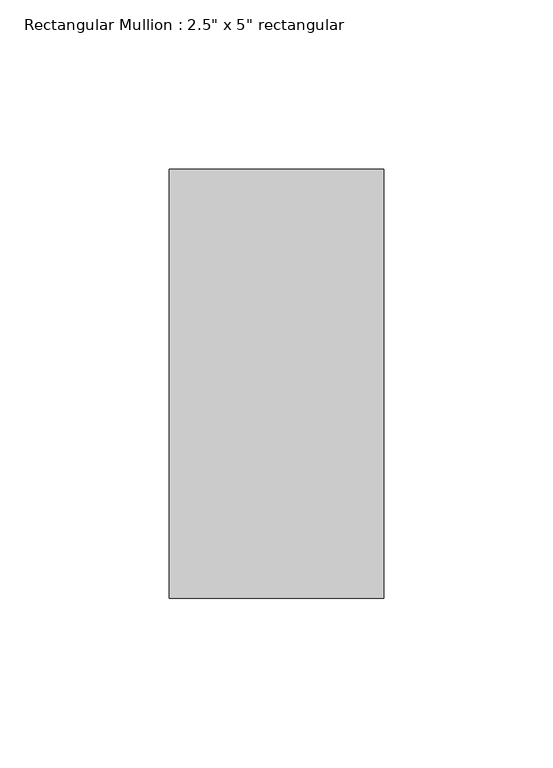
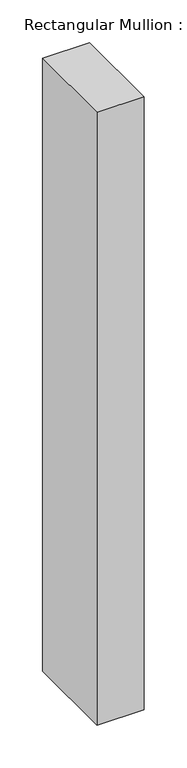
"""IFC4 building model written with IfcOpenShell, lengths in millimetres: member geometry."""

from ifc_helpers import new_model, si_unit, frame, origin, place, context, project, spatial, polyline, outline, extrude, source, transform, mapped, element, save


def member_f09d9db7(model_context):
    return source(origin(), model_context, "Body", "SweptSolid", [
        extrude(outline(polyline([(31.75, 63.5), (31.75, -63.5), (-31.75, -63.5), (-31.75, 63.5), (31.75, 63.5)])), frame((0.0, 0.0, -873.5902035), z_axis=(0.0, 0.0, 1.0), x_axis=(1.0, 0.0, 0.0)), (0.0, 0.0, 1.0), 873.5902035),
    ])


if __name__ == "__main__":
    model = new_model("IFC4")
    model_context = context("Model", 3, world=origin())
    ifc_project = project(units=[si_unit("LENGTHUNIT", "METRE", prefix="MILLI")], contexts=[model_context])
    site = spatial("IfcSite", under=ifc_project)
    building = spatial("IfcBuilding", under=site)
    placement = place(None, origin())
    member_shape = member_f09d9db7(model_context)
    element("IfcMember", 1, ObjectType="Rectangular Mullion : 2.5\" x 5\" rectangular", at=placement, inside=building, context=model_context, shape_type="MappedRepresentation", body=[
        mapped(member_shape, transform((0.0, 0.0, 0.0), x_axis=(1.0, 0.0, 0.0), y_axis=(0.0, 1.0, 0.0), z_axis=(0.0, 0.0, 1.0))),
    ])
    save(model, "model.ifc")

# Revit data of these elements
# Type "Rectangular Mullion : 2.5\" x 5\" rectangular"
#   built-in parameter 1007304 = 0.416667 (stored number, unit not read)
#   built-in parameter 1007301 = 0.104167 (stored number, unit not read)
#   built-in parameter 1007300 = 0.104167 (stored number, unit not read)
# Element 1 (IfcMember, "Rectangular Mullion : 2.5\" x 5\" rectangular")
#   Materials on its faces: "Aluminum"
# Materials
#   "Aluminum": class "Metal", colour RGB 247 247 247, transparency 0, Description = "Aluminum 6061", Cost = 0
